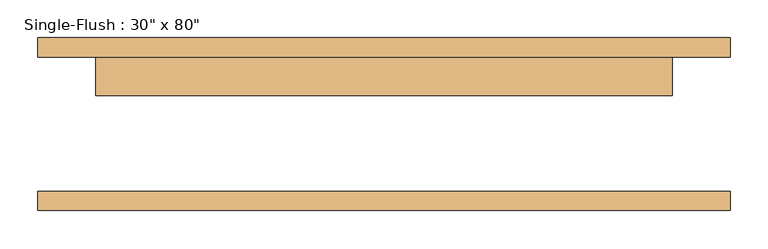
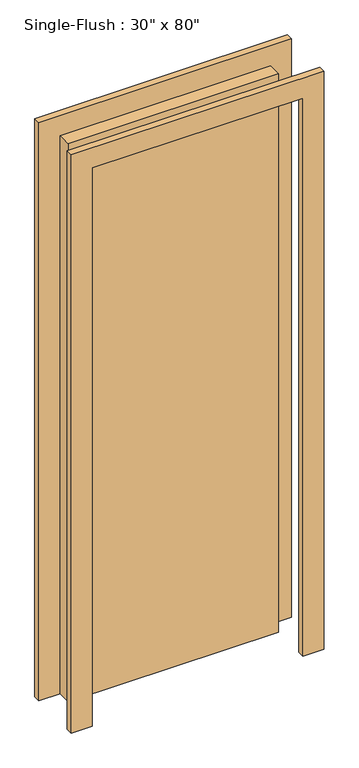
"""IFC4 building model written with IfcOpenShell, lengths in millimetres: door geometry."""

from ifc_helpers import new_model, si_unit, frame, origin, origin_with_axes, place, context, project, spatial, polyline, outline, extrude, source, transform, mapped, element, save


def door_0af0cdd0(model_context):
    return source(origin(), model_context, "Body", "SweptSolid", [
        extrude(outline(polyline([(2209.8, -457.2), (0.0, -457.2), (0.0, -381.0), (2133.6, -381.0), (2133.6, 381.0), (0.0, 381.0), (0.0, 457.2), (2209.8, 457.2), (2209.8, -457.2)])), frame((0.0, 88.9, 0.0), z_axis=(0.0, 1.0, 0.0), x_axis=(0.0, 0.0, 1.0)), (0.0, 0.0, 1.0), 25.4),
        extrude(outline(polyline([(2209.8, 457.2), (2209.8, -457.2), (0.0, -457.2), (0.0, -381.0), (2133.6, -381.0), (2133.6, 381.0), (0.0, 381.0), (0.0, 457.2), (2209.8, 457.2)])), frame((0.0, -114.3, 0.0), z_axis=(0.0, 1.0, 0.0), x_axis=(0.0, 0.0, 1.0)), (0.0, 0.0, 1.0), 25.4),
        extrude(outline(polyline([(381.0, 38.1), (-381.0, 38.1), (-381.0, 88.9), (381.0, 88.9), (381.0, 38.1)])), origin_with_axes(), (0.0, 0.0, 1.0), 2133.6),
    ])


if __name__ == "__main__":
    model = new_model("IFC4")
    model_context = context("Model", 3, world=origin())
    ifc_project = project(units=[si_unit("LENGTHUNIT", "METRE", prefix="MILLI")], contexts=[model_context])
    site = spatial("IfcSite", under=ifc_project)
    building = spatial("IfcBuilding", under=site)
    placement = place(None, origin())
    door_shape = door_0af0cdd0(model_context)
    element("IfcDoor", 1, ObjectType="Single-Flush : 30\" x 80\"", at=placement, inside=building, context=model_context, shape_type="MappedRepresentation", body=[
        mapped(door_shape, transform((0.0, 0.0, 0.0), x_axis=(1.0, 0.0, 0.0), y_axis=(0.0, 1.0, 0.0), z_axis=(0.0, 0.0, 1.0))),
    ])
    save(model, "model.ifc")

# Revit data of these elements
# Type "Single-Flush : 30\" x 80\""
#   Type Mark = "5"
#   Construction Type Id = "MDOOR"
#   Assembly Code = "C1020"
#   Analytic Construction = "Metal"
#   Thickness = 0' - 2"
#   Heat Transfer Coefficient (U) = 0.651978 BTU/(h·ft²·°F)
#   Height = 7' - 0"
#   Trim Projection Ext = 0' - 1"
#   Trim Projection Int = 0' - 1"
#   Trim Width = 0' - 3"
#   Width = 2' - 6"
#   Define Thermal Properties by = 1
#   Define Thermal Properties by = 1
#   Door Material = Door - Panel
#   Frame Material = Door - Frame
#   Visual Light Transmittance = 0
#   Solar Heat Gain Coefficient = 0
#   Function = (empty or 0)
#   Wall Closure = (empty or 0)
# Element 1 (IfcDoor, "Single-Flush : 30\" x 80\"")
#   Materials on its faces: "Door - Frame", "Door - Panel"
# Materials
#   "Door - Panel": class "Wood", colour RGB 210 159 95, transparency 0, Cost = 0
#   "Door - Frame": colour RGB 118 70 51, transparency 0, Cost = 0
